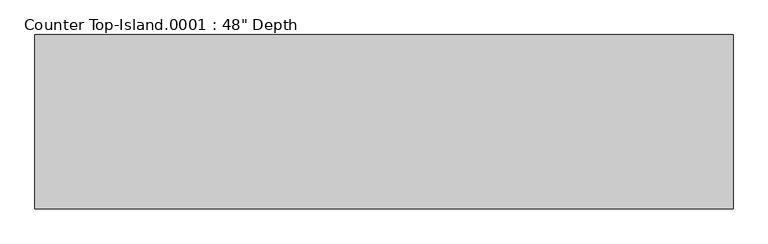
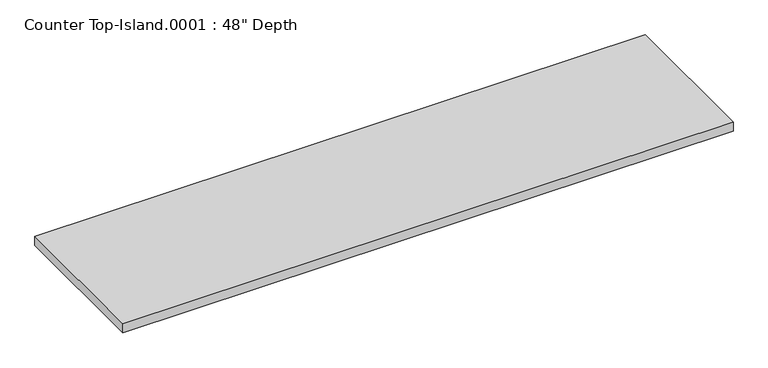
"""IFC4 building model written with IfcOpenShell, lengths in millimetres: furniture geometry."""

from ifc_helpers import new_model, si_unit, frame, origin, place, context, project, spatial, polyline, outline, extrude, source, transform, mapped, element, save


def furniture_15b2fe13(model_context):
    return source(origin(), model_context, "Body", "SweptSolid", [
        extrude(outline(polyline([(1237.9377049, 25.4), (1237.9377049, -584.2), (-1200.4622951, -584.2), (-1200.4622951, 25.4), (1237.9377049, 25.4)])), frame((0.0, 0.0, 876.3), z_axis=(0.0, 0.0, 1.0), x_axis=(1.0, 0.0, 0.0)), (0.0, 0.0, 1.0), 38.1),
    ])


if __name__ == "__main__":
    model = new_model("IFC4")
    model_context = context("Model", 3, world=origin())
    ifc_project = project(units=[si_unit("LENGTHUNIT", "METRE", prefix="MILLI")], contexts=[model_context])
    site = spatial("IfcSite", under=ifc_project)
    building = spatial("IfcBuilding", under=site)
    placement = place(None, origin())
    furniture_shape = furniture_15b2fe13(model_context)
    element("IfcFurniture", 1, ObjectType="Counter Top-Island.0001 : 48\" Depth", at=placement, inside=building, context=model_context, shape_type="MappedRepresentation", body=[
        mapped(furniture_shape, transform((0.0, 0.0, 0.0), x_axis=(1.0, 0.0, 0.0), y_axis=(0.0, 1.0, 0.0), z_axis=(0.0, 0.0, 1.0))),
    ])
    save(model, "model.ifc")

# Revit data of these elements
# Type "Counter Top-Island.0001 : 48\" Depth"
#   Assembly Code = "C1030400"
#   Width = 1' - 0"
#   Counter Thickness = 0' - 1 1/2"
#   Depth [instance default] = 4' - 2"
#   Height = 3' - 0"
#   Length [instance default] = 8' - 0"
#   Counter Top Material = none
#   Default Elevation = 0
# Element 1 (IfcFurniture, "Counter Top-Island.0001 : 48\" Depth")
#   Depth = 2' - 0"
#   Materials on its faces: "Counter Top"
# Materials
#   "Counter Top": class "Wood", colour RGB 226 177 128, transparency 0
